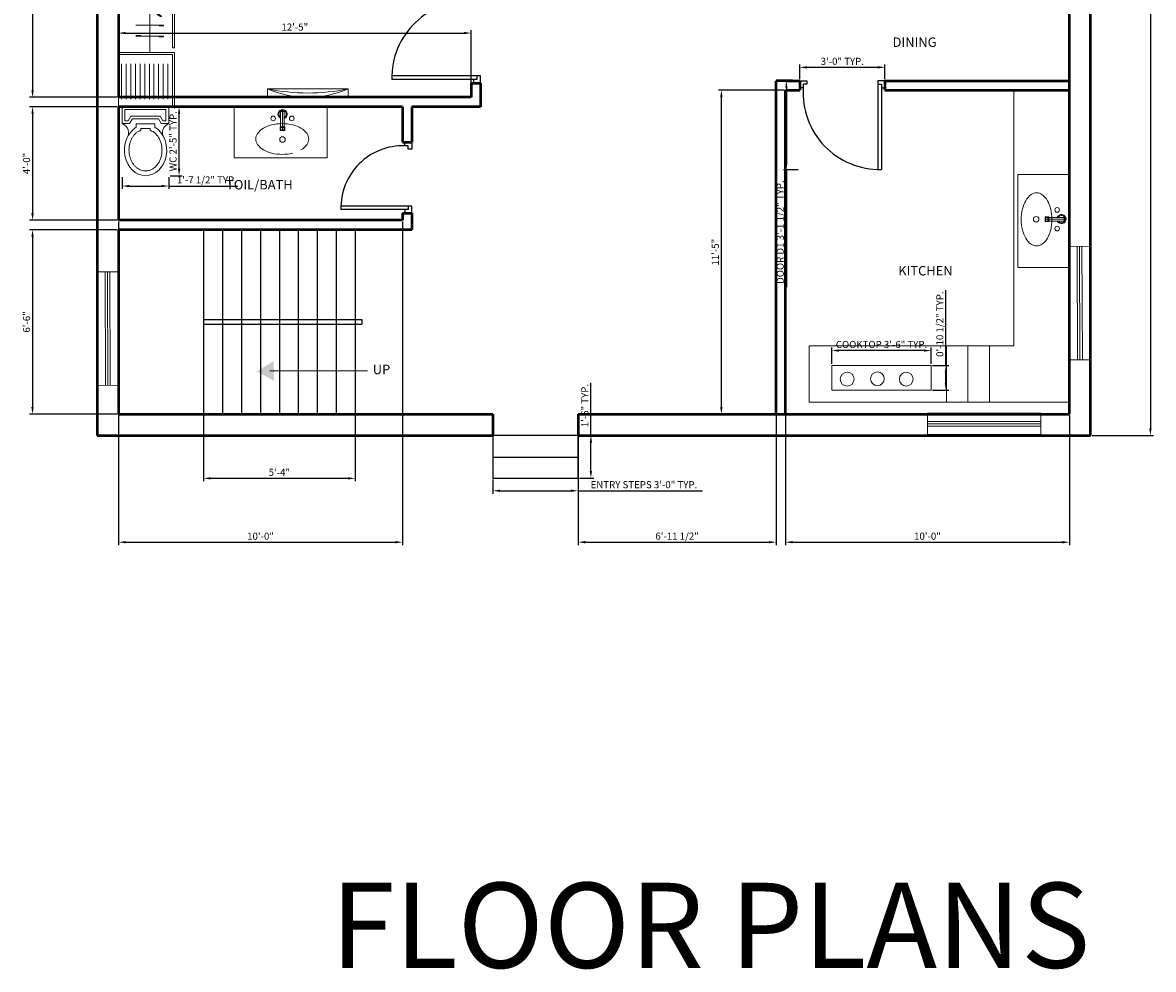
# Model space of a CAD drawing. Units: inches. Extents: x 108 to 1546, y -229 to 513.
# Tile 4 of 11: x 591 to 1070, y -229 to 171. Entities that reach past the tile are written whole.
import ezdxf

# ---------------------------------------------------------------- set-up
doc = ezdxf.new("R2010")
doc.units = ezdxf.units.IN
for name, color, linetype, lineweight in [('A-ANNO-DIMS', 2, 'Continuous', 18), ('A-ANNO-SYMB', 4, 'Continuous', 18), ('A-AREA-IDEN', 4, 'Continuous', 18), ('A-EQPM', 8, 'Continuous', 18), ('A-FLOR-CBNT', 8, 'Continuous', 18), ('A-FLOR-FIXT', 9, 'Continuous', 18), ('A-FLOR-STRS', 7, 'Continuous', 25), ('A-FURN', 8, 'Continuous', 13), ('door', 1, 'Continuous', 25), ('tv', 2, 'Continuous', 13), ('wall', 7, 'Continuous', 50), ('WINDOW', 212, 'Continuous', 18)]:
    doc.layers.add(name, color=color, linetype=linetype, lineweight=lineweight)
doc.layers.add('A-ANNO-TEXT', color=30, linetype='Continuous', lineweight=35, true_color=0xf26722)
doc.styles.get("Standard").update_dxf_attribs({"font": 'arial.ttf'})
doc.dimstyles.new('ISO-25', dxfattribs={"dimtxt": 3, "dimasz": 3, "dimexe": 1.25, "dimexo": 0.625, "dimtad": 1, "dimdec": 1, "dimlunit": 3, "dimtxsty": 'Standard', "dimcen": 2.5, "dimadec": 0, "dimazin": 0, "dimtfac": 1, "dimtdec": 1, "dimtmove": 0, "dimatfit": 3, "dimfxl": 1, "dimarcsym": 0})

# ---------------------------------------------------------------- blocks, each defined once
blk = doc.blocks.new('A$C50A015BB')
for p, q in [((0, 0.55), (1, 0.55)), ((0, 0.55), (0, 0)), ((0.498, 0.5), (0.538, 0.5)), ((0.498, 0.5), (0.498, 0.3)), ((0.518, 0.5), (0.518, 0.3)), ((0.538, 0.5), (0.538, 0.3)), ((1, 0.55), (1, 0)), ((0.493, 0.335), (0.493, 0.295)), ((0.493, 0.335), (0.543, 0.335)), ((0.493, 0.295), (0.543, 0.295)), ((0.498, 0.325), (0.538, 0.325)), ((0.498, 0.3), (0.538, 0.3)), ((0.543, 0.335), (0.543, 0.295)), ((0, 0), (1, 0)), ((0, 0), (1, 0))]:
    blk.add_line(p, q)
for centre, radius in [((0.418, 0.424), 0.025), ((0.618, 0.424), 0.025), ((0.518, 0.198), 0.0298)]:
    blk.add_circle(centre, radius)
for centre, radius, start, end in [((0.52, 0.47), 0.0497, 291.7425, 244.2331), ((0.52, 0.47), 0.0397, 297.632, 237.0256), ((0.516, -0.123), 0.491, 90, 103.4853), ((0.516, -0.123), 0.491, 76.5147, 90), ((0.33, 0.203), 0.0991, 144.4178, 180), ((0.418, 0.14), 0.208, 120.0686, 144.4178), ((0.477, 0.038), 0.325, 103.4853, 120.0686), ((0.554, 0.038), 0.325, 59.9314, 76.5147), ((0.613, 0.14), 0.208, 35.5822, 59.9314), ((0.702, 0.203), 0.0991, 0, 35.5822), ((0.33, 0.203), 0.0991, 180, 215.5822), ((0.418, 0.267), 0.208, 215.5822, 239.9314), ((0.613, 0.267), 0.208, 300.0686, 324.4178), ((0.702, 0.203), 0.0991, 324.4178, 0), ((0.477, 0.368), 0.325, 239.9314, 256.5147), ((0.516, 0.529), 0.491, 256.5147, 270), ((0.516, 0.529), 0.491, 270, 283.4853), ((0.554, 0.368), 0.325, 283.4853, 300.0686)]:
    blk.add_arc(centre, radius, start, end)
blk = doc.blocks.new('A$C7C8779AE')
for p, q in [((0, 0.74), (0, 0.56)), ((0.5, 0.74), (0, 0.74)), ((0.5, 0.56), (0.5, 0.74)), ((0.47, 0.71), (0.03, 0.71)), ((0.03, 0.71), (0.03, 0.59)), ((0.093, 0.64), (0.063, 0.59)), ((0.11, 0.61), (0.08, 0.56)), ((0.093, 0.64), (0.407, 0.64)), ((0.11, 0.61), (0.39, 0.61)), ((0.42, 0.56), (0.39, 0.61)), ((0.437, 0.59), (0.407, 0.64)), ((0.47, 0.59), (0.47, 0.71)), ((0, 0.56), (0.08, 0.56)), ((0.03, 0.59), (0.063, 0.59)), ((0.15, 0.557), (0.15, 0.52)), ((0.15, 0.557), (0.351, 0.557)), ((0.2, 0.507), (0.2, 0.488)), ((0.2, 0.507), (0.301, 0.507)), ((0.301, 0.507), (0.301, 0.488)), ((0.351, 0.557), (0.351, 0.52)), ((0.42, 0.56), (0.5, 0.56)), ((0.437, 0.59), (0.47, 0.59))]:
    blk.add_line(p, q)
for centre, start, end in [((-0.039, 0.461), 344.642, 68.7339), ((0.539, 0.461), 111.2661, 195.358)]:
    blk.add_arc(centre, 0.106, start, end)
blk.add_ellipse((0.251, 0.274), major_axis=(0, 0.274), ratio=0.828948, start_param=0.459479, end_param=5.823706)
blk.add_open_spline([(0.2, 0.488), (0.17, 0.474), (0.164, 0.47), (0.151, 0.46), (0.144, 0.454), (0.13, 0.439), (0.123, 0.431), (0.111, 0.413), (0.106, 0.404), (0.096, 0.384), (0.091, 0.373), (0.084, 0.352), (0.081, 0.34), (0.076, 0.317), (0.075, 0.305), (0.073, 0.282), (0.073, 0.27), (0.074, 0.246), (0.076, 0.234), (0.08, 0.211), (0.083, 0.2), (0.09, 0.178), (0.095, 0.167), (0.104, 0.147), (0.11, 0.138), (0.122, 0.12), (0.128, 0.112), (0.142, 0.097), (0.149, 0.09), (0.165, 0.078), (0.173, 0.073), (0.189, 0.064), (0.197, 0.06), (0.214, 0.055), (0.222, 0.053), (0.239, 0.05), (0.248, 0.05), (0.266, 0.051), (0.276, 0.052), (0.296, 0.057), (0.306, 0.061), (0.325, 0.071), (0.335, 0.077), (0.353, 0.091), (0.361, 0.099), (0.377, 0.117), (0.384, 0.127), (0.398, 0.149), (0.404, 0.161), (0.414, 0.185), (0.418, 0.198), (0.424, 0.225), (0.426, 0.239), (0.428, 0.267), (0.428, 0.281), (0.426, 0.309), (0.424, 0.323), (0.418, 0.349), (0.414, 0.363), (0.404, 0.387), (0.398, 0.399), (0.385, 0.421), (0.378, 0.431), (0.362, 0.449), (0.353, 0.458), (0.338, 0.469), (0.332, 0.474), (0.301, 0.488)], degree=3, knots=[0.459479, 0.459479, 0.459479, 0.459479, 0.567422, 0.567422, 0.720865, 0.720865, 0.874307, 0.874307, 1.02775, 1.02775, 1.181192, 1.181192, 1.334635, 1.334635, 1.488077, 1.488077, 1.64152, 1.64152, 1.794963, 1.794963, 1.948405, 1.948405, 2.101848, 2.101848, 2.25529, 2.25529, 2.408733, 2.408733, 2.562175, 2.562175, 2.715618, 2.715618, 2.86906, 2.86906, 3.022503, 3.022503, 3.175946, 3.175946, 3.356457, 3.356457, 3.536968, 3.536968, 3.717479, 3.717479, 3.89799, 3.89799, 4.078501, 4.078501, 4.259012, 4.259012, 4.439523, 4.439523, 4.620035, 4.620035, 4.800546, 4.800546, 4.981057, 4.981057, 5.161568, 5.161568, 5.342079, 5.342079, 5.52259, 5.52259, 5.703101, 5.703101, 5.823706, 5.823706, 5.823706, 5.823706])
blk = doc.blocks.new('A$C34930FF8')
at = {"ltscale": 0.05}
for p, q in [((0, 2252), (0, 17)), ((600, 2252), (0, 2252)), ((185, 1513), (185, 1521)), ((227, 1479), (233, 1485)), ((238, 1513), (238, 1521)), ((437, 1513), (437, 1504)), ((482, 1513), (482, 1504)), ((264, 1442), (270, 1448)), ((185, 1229), (185, 1238)), ((238, 1229), (238, 1238)), ((398, 1304), (392, 1298)), ((435, 1266), (429, 1260)), ((437, 1228), (437, 1220)), ((482, 1228), (482, 1220)), ((209, 1150), (214, 1157)), ((253, 1122), (258, 1129)), ((415, 1018), (411, 1010)), ((459, 989), (455, 982)), ((482, 895), (482, 886)), ((238, 775), (238, 784)), ((437, 775), (437, 767)), ((482, 775), (482, 767)), ((600, 17), (0, 17))]:
    blk.add_line(p, q, dxfattribs=at)
for p, q in [((580, 1691), (580, 2252)), ((600, 1669), (600, 2269)), ((30, 1791), (30, 2169)), ((80, 1791), (80, 2169)), ((130, 1791), (130, 2169)), ((180, 1791), (180, 2169)), ((230, 1791), (230, 2169)), ((280, 1791), (280, 2169)), ((330, 1791), (330, 2169)), ((380, 1791), (380, 2169)), ((430, 1791), (430, 2169)), ((480, 1791), (480, 2169)), ((530, 1791), (530, 2169)), ((580, 1691), (0, 1691)), ((600, 1669), (0, 1669)), ((335, 1666), (335, 603)), ((600, 1603), (620, 1603)), ((600, 1019), (600, 1603)), ((620, 1603), (620, 1019)), ((238, 1521), (185, 1521)), ((482, 1513), (185, 1513)), ((435, 1266), (227, 1479)), ((270, 1448), (233, 1485)), ((437, 1504), (482, 1504)), ((238, 1238), (185, 1238)), ((482, 1228), (185, 1228)), ((429, 1260), (392, 1298)), ((437, 1220), (482, 1220)), ((600, 1233), (580, 1233)), ((580, 1233), (580, 649)), ((600, 649), (600, 1233)), ((459, 989), (209, 1150)), ((258, 1129), (214, 1157)), ((455, 982), (411, 1010)), ((620, 1019), (600, 1019)), ((482, 895), (185, 895)), ((437, 886), (482, 886)), ((238, 784), (185, 784)), ((482, 775), (185, 775)), ((437, 767), (482, 767)), ((580, 649), (600, 649)), ((600, 600), (0, 600)), ((580, 578), (0, 578)), ((580, 578), (580, 17)), ((600, 600), (600, 0)), ((30, 478), (30, 100)), ((80, 478), (80, 100)), ((130, 478), (130, 100)), ((180, 478), (180, 100)), ((230, 478), (230, 100)), ((280, 478), (280, 100)), ((330, 478), (330, 100)), ((380, 478), (380, 100)), ((430, 478), (430, 100)), ((480, 478), (480, 100)), ((530, 478), (530, 100))]:
    blk.add_line(p, q)
blk = doc.blocks.new('*D24')
at = {"layer": 'A-ANNO-DIMS', "color": 0, "lineweight": -2, "transparency": 16777216}
for p, q in [((1043.62, 476.47), (1069.53, 476.47)), ((1068.28, 473.47), (1068.28, -0.53)), ((1043.62, -3.53), (1069.53, -3.53))]:
    blk.add_line(p, q, dxfattribs=at)
at = {"layer": 'A-ANNO-DIMS', "color": 0, "transparency": 16777216}
for points in [[(1067.78, 473.47), (1068.78, 473.47), (1068.28, 476.47)], [(1067.78, -0.53), (1068.78, -0.53), (1068.28, -3.53)]]:
    blk.add_solid(points, dxfattribs=at)
at = {"layer": 'Defpoints', "color": 0, "transparency": 16777216}
for p in [(1043, 476.47), (1043, -3.53), (1068.28, -3.53)]:
    blk.add_point(p, dxfattribs=at)
at = {"layer": 'A-ANNO-DIMS', "color": 0, "transparency": 16777216, "insert": (1066.12, 236.47), "char_height": 3, "attachment_point": 5, "rotation": 90}
blk.add_mtext("40'", dxfattribs=at)
blk = doc.blocks.new('WINDOW-48X9')
for p, q in [((0, 9), (0, 0)), ((0, 9), (48, 9)), ((0, 5.5), (48, 5.5)), ((48, 9), (48, 0)), ((0, 4.5), (48, 4.5)), ((0, 3.5), (48, 3.5)), ((0, 0), (48, 0))]:
    blk.add_line(p, q)
blk = doc.blocks.new('DOOR-SWING-36')
for p, q in [((1.5, 1.5), (1.5, 37.5)), ((3, 1.5), (3, 37.5)), ((0, 3), (0, 0)), ((1.5, 3), (0, 3)), ((1.5, 1.5), (1.5, 3)), ((3, 1.5), (1.5, 1.5)), ((3, 0), (3, 1.5)), ((33, 0), (33, 1.5)), ((33, 1.5), (34.5, 1.5)), ((34.5, 1.5), (34.5, 3)), ((34.5, 3), (36, 3)), ((36, 3), (36, 0)), ((0, 0), (3, 0)), ((36, 0), (33, 0))]:
    blk.add_line(p, q)
blk.add_arc((2.25, 5.18), 32.32, 356.1244, 91.3295)
blk = doc.blocks.new('DOOR-SWING-30')
for p, q in [((27, 30), (30, 30)), ((27, 28.5), (27, 30)), ((30, 30), (30, 27)), ((28.5, 28.5), (27, 28.5)), ((28.5, 27), (28.5, 28.5)), ((30, 27), (28.5, 27)), ((30, 3), (0, 3)), ((28.5, 1.5), (0, 1.5)), ((28.5, 1.5), (27, 1.5)), ((27, 1.5), (27, 0)), ((30, 3), (28.5, 3)), ((28.5, 3), (28.5, 1.5)), ((30, 0), (30, 3)), ((27, 0), (30, 0))]:
    blk.add_line(p, q)
blk.add_arc((26.25, 2.25), 26.26, 88.3634, 181.6366)
blk = doc.blocks.new('TV-WALL-MOUNT')
blk.add_lwpolyline([(0, 0), (34.19, 0), (34.19, 3.56), (0, 3.56)], close=True)
for centre, radius, start, end in [((17.1, 42.8), 42.8, 246.4582, 293.5418), ((17.1, 84.72), 82.93, 258.1036, 281.8964)]:
    blk.add_arc(centre, radius, start, end)
blk = doc.blocks.new('COOKTOP-3-BURNER')
blk.add_lwpolyline([(0, 41.89), (10.48, 41.89), (10.48, 0), (0, 0)], close=True)
for centre in [(4.66, 35.46), (4.81, 22.66), (4.66, 10.45)]:
    blk.add_circle(centre, 2.9)
blk = doc.blocks.new('COUNTER-INSERT-DIVIDED')
blk.add_line((0, 9.14), (23.96, 9.14))
blk.add_lwpolyline([(0, 18.28), (23.96, 18.28), (23.96, 0), (0, 0)], close=True)
blk = doc.blocks.new('ENTRY-STEPS-36')
for p, q in [((0, 8.79), (36, 8.79)), ((0, 0), (36, 0))]:
    blk.add_line(p, q)
blk.add_lwpolyline([(36, 0), (36, 18), (0, 18), (0, 0)])
blk = doc.blocks.new('*D38')
at = {"layer": 'A-ANNO-DIMS', "color": 0, "lineweight": -2, "transparency": 16777216}
for p, q in [((919.37, 146.47), (913.09, 146.47)), ((914.34, 143.47), (914.34, 111.76)), ((919.37, 108.76), (913.09, 108.76)), ((914.34, 108.76), (914.34, 59.12))]:
    blk.add_line(p, q, dxfattribs=at)
at = {"layer": 'A-ANNO-DIMS', "color": 0, "transparency": 16777216}
for points in [[(913.84, 143.47), (914.84, 143.47), (914.34, 146.47)], [(913.84, 111.76), (914.84, 111.76), (914.34, 108.76)]]:
    blk.add_solid(points, dxfattribs=at)
at = {"layer": 'Defpoints', "color": 0, "transparency": 16777216}
for p in [(920, 146.47), (914.34, 108.76), (920, 108.76)]:
    blk.add_point(p, dxfattribs=at)
at = {"layer": 'A-ANNO-DIMS', "color": 0, "transparency": 16777216, "insert": (912.16, 82.44), "char_height": 3, "attachment_point": 5, "rotation": 90}
blk.add_mtext('DOOR D1 3\'-1 1/2" TYP.', dxfattribs=at)
blk = doc.blocks.new('*D39')
at = {"layer": 'A-ANNO-DIMS', "color": 0, "lineweight": -2, "transparency": 16777216}
for p, q in [((920, 147.09), (920, 153.38)), ((956, 147.09), (956, 153.38)), ((953, 152.13), (923, 152.13))]:
    blk.add_line(p, q, dxfattribs=at)
at = {"layer": 'A-ANNO-DIMS', "color": 0, "transparency": 16777216}
for points in [[(923, 152.63), (923, 151.63), (920, 152.13)], [(953, 152.63), (953, 151.63), (956, 152.13)]]:
    blk.add_solid(points, dxfattribs=at)
at = {"layer": 'Defpoints', "color": 0, "transparency": 16777216}
for p in [(920, 152.13), (920, 146.47), (956, 146.47)]:
    blk.add_point(p, dxfattribs=at)
at = {"layer": 'A-ANNO-DIMS', "color": 0, "transparency": 16777216, "insert": (938, 154.28), "char_height": 3, "attachment_point": 5}
blk.add_mtext('3\'-0" TYP.', dxfattribs=at)
blk = doc.blocks.new('*D48')
at = {"layer": 'A-ANNO-DIMS', "color": 0, "lineweight": -2, "transparency": 16777216}
for p, q in [((653.82, 135.47), (658.82, 135.47)), ((657.57, 109.32), (657.57, 132.47)), ((653.82, 106.32), (658.82, 106.32))]:
    blk.add_line(p, q, dxfattribs=at)
at = {"layer": 'A-ANNO-DIMS', "color": 0, "transparency": 16777216}
for points in [[(657.07, 132.47), (658.07, 132.47), (657.57, 135.47)], [(657.07, 109.32), (658.07, 109.32), (657.57, 106.32)]]:
    blk.add_solid(points, dxfattribs=at)
at = {"layer": 'Defpoints', "color": 0, "transparency": 16777216}
for p in [(653.2, 135.47), (657.57, 135.47), (653.2, 106.32)]:
    blk.add_point(p, dxfattribs=at)
at = {"layer": 'A-ANNO-DIMS', "color": 0, "transparency": 16777216, "insert": (655.4, 120.89), "char_height": 3, "attachment_point": 5, "rotation": 90}
blk.add_mtext('WC 2\'-5" TYP.', dxfattribs=at)
blk = doc.blocks.new('*D49')
at = {"layer": 'A-ANNO-DIMS', "color": 0, "lineweight": -2, "transparency": 16777216}
for p, q in [((633.51, 105.69), (633.51, 100.7)), ((653.2, 105.69), (653.2, 100.7)), ((636.51, 101.95), (650.2, 101.95)), ((653.2, 101.95), (682.44, 101.95))]:
    blk.add_line(p, q, dxfattribs=at)
at = {"layer": 'A-ANNO-DIMS', "color": 0, "transparency": 16777216}
for points in [[(636.51, 102.45), (636.51, 101.45), (633.51, 101.95)], [(650.2, 102.45), (650.2, 101.45), (653.2, 101.95)]]:
    blk.add_solid(points, dxfattribs=at)
at = {"layer": 'Defpoints', "color": 0, "transparency": 16777216}
for p in [(633.51, 106.32), (653.2, 106.32), (653.2, 101.95)]:
    blk.add_point(p, dxfattribs=at)
at = {"layer": 'A-ANNO-DIMS', "color": 0, "transparency": 16777216, "insert": (669.32, 104.12), "char_height": 3, "attachment_point": 5}
blk.add_mtext('1\'-7 1/2" TYP.', dxfattribs=at)
blk = doc.blocks.new('*D62')
at = {"layer": 'A-ANNO-DIMS', "color": 0, "lineweight": -2, "transparency": 16777216}
for p, q in [((933.62, 26.71), (933.62, 33.62)), ((975.51, 26.71), (975.51, 33.62)), ((972.51, 32.37), (936.62, 32.37))]:
    blk.add_line(p, q, dxfattribs=at)
at = {"layer": 'A-ANNO-DIMS', "color": 0, "transparency": 16777216}
for points in [[(936.62, 32.87), (936.62, 31.87), (933.62, 32.37)], [(972.51, 32.87), (972.51, 31.87), (975.51, 32.37)]]:
    blk.add_solid(points, dxfattribs=at)
at = {"layer": 'Defpoints', "color": 0, "transparency": 16777216}
for p in [(933.62, 32.37), (933.62, 26.09), (975.51, 26.09)]:
    blk.add_point(p, dxfattribs=at)
at = {"layer": 'A-ANNO-DIMS', "color": 0, "transparency": 16777216, "insert": (954.57, 34.55), "char_height": 3, "attachment_point": 5}
blk.add_mtext('COOKTOP 3\'-6" TYP.', dxfattribs=at)
blk = doc.blocks.new('*D63')
at = {"layer": 'A-ANNO-DIMS', "color": 0, "lineweight": -2, "transparency": 16777216}
for p, q in [((981.8, 26.09), (981.8, 57.95)), ((976.14, 26.09), (983.05, 26.09)), ((981.8, 18.61), (981.8, 23.09)), ((976.14, 15.61), (983.05, 15.61))]:
    blk.add_line(p, q, dxfattribs=at)
at = {"layer": 'A-ANNO-DIMS', "color": 0, "transparency": 16777216}
for points in [[(981.3, 23.09), (982.3, 23.09), (981.8, 26.09)], [(981.3, 18.61), (982.3, 18.61), (981.8, 15.61)]]:
    blk.add_solid(points, dxfattribs=at)
at = {"layer": 'Defpoints', "color": 0, "transparency": 16777216}
for p in [(975.51, 26.09), (981.8, 26.09), (975.51, 15.61)]:
    blk.add_point(p, dxfattribs=at)
at = {"layer": 'A-ANNO-DIMS', "color": 0, "transparency": 16777216, "insert": (979.62, 43.52), "char_height": 3, "attachment_point": 5, "rotation": 90}
blk.add_mtext('0\'-10 1/2" TYP.', dxfattribs=at)
blk = doc.blocks.new('*D66')
at = {"layer": 'A-ANNO-DIMS', "color": 0, "lineweight": -2, "transparency": 16777216}
for p, q in [((790.29, -22.16), (790.29, -28.18)), ((826.29, -22.16), (826.29, -28.18)), ((793.29, -26.93), (823.29, -26.93)), ((826.29, -26.93), (878.94, -26.93))]:
    blk.add_line(p, q, dxfattribs=at)
at = {"layer": 'A-ANNO-DIMS', "color": 0, "transparency": 16777216}
for points in [[(793.29, -26.43), (793.29, -27.43), (790.29, -26.93)], [(823.29, -26.43), (823.29, -27.43), (826.29, -26.93)]]:
    blk.add_solid(points, dxfattribs=at)
at = {"layer": 'Defpoints', "color": 0, "transparency": 16777216}
for p in [(790.29, -21.53), (826.29, -21.53), (826.29, -26.93)]:
    blk.add_point(p, dxfattribs=at)
at = {"layer": 'A-ANNO-DIMS', "color": 0, "transparency": 16777216, "insert": (854.11, -24.75), "char_height": 3, "attachment_point": 5}
blk.add_mtext('ENTRY STEPS 3\'-0" TYP.', dxfattribs=at)
blk = doc.blocks.new('*D67')
at = {"layer": 'A-ANNO-DIMS', "color": 0, "lineweight": -2, "transparency": 16777216}
for p, q in [((831.69, -3.53), (831.69, 18.72)), ((826.91, -3.53), (832.94, -3.53)), ((831.69, -18.53), (831.69, -6.53)), ((826.91, -21.53), (832.94, -21.53))]:
    blk.add_line(p, q, dxfattribs=at)
at = {"layer": 'A-ANNO-DIMS', "color": 0, "transparency": 16777216}
for points in [[(831.19, -6.53), (832.19, -6.53), (831.69, -3.53)], [(831.19, -18.53), (832.19, -18.53), (831.69, -21.53)]]:
    blk.add_solid(points, dxfattribs=at)
at = {"layer": 'Defpoints', "color": 0, "transparency": 16777216}
for p in [(826.29, -3.53), (831.69, -3.53), (826.29, -21.53)]:
    blk.add_point(p, dxfattribs=at)
at = {"layer": 'A-ANNO-DIMS', "color": 0, "transparency": 16777216, "insert": (829.53, 9.1), "char_height": 3, "attachment_point": 5, "rotation": 90}
blk.add_mtext('1\'-6" TYP.', dxfattribs=at)
blk = doc.blocks.new('*D87')
at = {"layer": 'A-ANNO-DIMS', "color": 0, "lineweight": -2, "transparency": 16777216}
for p, q in [((632, 86.84), (632, -49.93)), ((752, 86.84), (752, -49.93)), ((635, -48.68), (749, -48.68))]:
    blk.add_line(p, q, dxfattribs=at)
at = {"layer": 'A-ANNO-DIMS', "color": 0, "transparency": 16777216}
for points in [[(635, -48.18), (635, -49.18), (632, -48.68)], [(749, -48.18), (749, -49.18), (752, -48.68)]]:
    blk.add_solid(points, dxfattribs=at)
at = {"layer": 'Defpoints', "color": 0, "transparency": 16777216}
for p in [(632, 87.47), (752, 87.47), (752, -48.68)]:
    blk.add_point(p, dxfattribs=at)
at = {"layer": 'A-ANNO-DIMS', "color": 0, "transparency": 16777216, "insert": (692, -46.52), "char_height": 3, "attachment_point": 5}
blk.add_mtext('10\'-0"', dxfattribs=at)
blk = doc.blocks.new('*D88')
at = {"layer": 'A-ANNO-DIMS', "color": 0, "lineweight": -2, "transparency": 16777216}
for p, q in [((632, 140.09), (632, 167.87)), ((781, 140.09), (781, 167.87)), ((635, 166.62), (778, 166.62))]:
    blk.add_line(p, q, dxfattribs=at)
at = {"layer": 'A-ANNO-DIMS', "color": 0, "transparency": 16777216}
for points in [[(635, 167.12), (635, 166.12), (632, 166.62)], [(778, 167.12), (778, 166.12), (781, 166.62)]]:
    blk.add_solid(points, dxfattribs=at)
at = {"layer": 'Defpoints', "color": 0, "transparency": 16777216}
for p in [(781, 166.62), (632, 139.47), (781, 139.47)]:
    blk.add_point(p, dxfattribs=at)
at = {"layer": 'A-ANNO-DIMS', "color": 0, "transparency": 16777216, "insert": (706.5, 168.78), "char_height": 3, "attachment_point": 5}
blk.add_mtext('12\'-5"', dxfattribs=at)
blk = doc.blocks.new('*D89')
at = {"layer": 'A-ANNO-DIMS', "color": 0, "lineweight": -2, "transparency": 16777216}
for p, q in [((914, 4.84), (914, -49.93)), ((1034, 4.84), (1034, -49.93)), ((917, -48.68), (1031, -48.68))]:
    blk.add_line(p, q, dxfattribs=at)
at = {"layer": 'A-ANNO-DIMS', "color": 0, "transparency": 16777216}
for points in [[(917, -48.18), (917, -49.18), (914, -48.68)], [(1031, -48.18), (1031, -49.18), (1034, -48.68)]]:
    blk.add_solid(points, dxfattribs=at)
at = {"layer": 'Defpoints', "color": 0, "transparency": 16777216}
for p in [(914, 5.47), (1034, 5.47), (1034, -48.68)]:
    blk.add_point(p, dxfattribs=at)
at = {"layer": 'A-ANNO-DIMS', "color": 0, "transparency": 16777216, "insert": (974, -46.52), "char_height": 3, "attachment_point": 5}
blk.add_mtext('10\'-0"', dxfattribs=at)
blk = doc.blocks.new('*D90')
at = {"layer": 'A-ANNO-DIMS', "color": 0, "lineweight": -2, "transparency": 16777216}
for p, q in [((910, 4.84), (910, -49.93)), ((826.29, -4.16), (826.29, -49.93)), ((829.29, -48.68), (907, -48.68))]:
    blk.add_line(p, q, dxfattribs=at)
at = {"layer": 'A-ANNO-DIMS', "color": 0, "transparency": 16777216}
for points in [[(829.29, -48.18), (829.29, -49.18), (826.29, -48.68)], [(907, -48.18), (907, -49.18), (910, -48.68)]]:
    blk.add_solid(points, dxfattribs=at)
at = {"layer": 'Defpoints', "color": 0, "transparency": 16777216}
for p in [(910, 5.47), (826.29, -3.53), (910, -48.68)]:
    blk.add_point(p, dxfattribs=at)
at = {"layer": 'A-ANNO-DIMS', "color": 0, "transparency": 16777216, "insert": (868.14, -46.5), "char_height": 3, "attachment_point": 5}
blk.add_mtext('6\'-11 1/2"', dxfattribs=at)
blk = doc.blocks.new('*D93')
at = {"layer": 'A-ANNO-DIMS', "color": 0, "lineweight": -2, "transparency": 16777216}
for p, q in [((631.37, 307.47), (594.36, 307.47)), ((595.61, 304.47), (595.61, 142.47)), ((631.37, 139.47), (594.36, 139.47))]:
    blk.add_line(p, q, dxfattribs=at)
at = {"layer": 'A-ANNO-DIMS', "color": 0, "transparency": 16777216}
for points in [[(595.11, 304.47), (596.11, 304.47), (595.61, 307.47)], [(595.11, 142.47), (596.11, 142.47), (595.61, 139.47)]]:
    blk.add_solid(points, dxfattribs=at)
at = {"layer": 'Defpoints', "color": 0, "transparency": 16777216}
for p in [(632, 307.47), (595.61, 139.47), (632, 139.47)]:
    blk.add_point(p, dxfattribs=at)
at = {"layer": 'A-ANNO-DIMS', "color": 0, "transparency": 16777216, "insert": (593.45, 223.47), "char_height": 3, "attachment_point": 5, "rotation": 90}
blk.add_mtext('14\'-0"', dxfattribs=at)
blk = doc.blocks.new('*D94')
at = {"layer": 'A-ANNO-DIMS', "color": 0, "lineweight": -2, "transparency": 16777216}
for p, q in [((631.37, 135.47), (594.36, 135.47)), ((595.61, 132.47), (595.61, 90.47)), ((631.37, 87.47), (594.36, 87.47))]:
    blk.add_line(p, q, dxfattribs=at)
at = {"layer": 'A-ANNO-DIMS', "color": 0, "transparency": 16777216}
for points in [[(595.11, 132.47), (596.11, 132.47), (595.61, 135.47)], [(595.11, 90.47), (596.11, 90.47), (595.61, 87.47)]]:
    blk.add_solid(points, dxfattribs=at)
at = {"layer": 'Defpoints', "color": 0, "transparency": 16777216}
for p in [(632, 135.47), (595.61, 87.47), (632, 87.47)]:
    blk.add_point(p, dxfattribs=at)
at = {"layer": 'A-ANNO-DIMS', "color": 0, "transparency": 16777216, "insert": (593.45, 111.47), "char_height": 3, "attachment_point": 5, "rotation": 90}
blk.add_mtext('4\'-0"', dxfattribs=at)
blk = doc.blocks.new('*D95')
at = {"layer": 'A-ANNO-DIMS', "color": 0, "lineweight": -2, "transparency": 16777216}
for p, q in [((631.37, 83.47), (594.36, 83.47)), ((595.61, 80.47), (595.61, 8.47)), ((631.37, 5.47), (594.36, 5.47))]:
    blk.add_line(p, q, dxfattribs=at)
at = {"layer": 'A-ANNO-DIMS', "color": 0, "transparency": 16777216}
for points in [[(595.11, 80.47), (596.11, 80.47), (595.61, 83.47)], [(595.11, 8.47), (596.11, 8.47), (595.61, 5.47)]]:
    blk.add_solid(points, dxfattribs=at)
at = {"layer": 'Defpoints', "color": 0, "transparency": 16777216}
for p in [(632, 83.47), (595.61, 5.47), (632, 5.47)]:
    blk.add_point(p, dxfattribs=at)
at = {"layer": 'A-ANNO-DIMS', "color": 0, "transparency": 16777216, "insert": (593.45, 44.47), "char_height": 3, "attachment_point": 5, "rotation": 90}
blk.add_mtext('6\'-6"', dxfattribs=at)
blk = doc.blocks.new('*D96')
at = {"layer": 'A-ANNO-DIMS', "color": 0, "lineweight": -2, "transparency": 16777216}
for p, q in [((913.37, 142.47), (885.6, 142.47)), ((886.85, 8.47), (886.85, 139.47)), ((913.37, 5.47), (885.6, 5.47))]:
    blk.add_line(p, q, dxfattribs=at)
at = {"layer": 'A-ANNO-DIMS', "color": 0, "transparency": 16777216}
for points in [[(886.35, 139.47), (887.35, 139.47), (886.85, 142.47)], [(886.35, 8.47), (887.35, 8.47), (886.85, 5.47)]]:
    blk.add_solid(points, dxfattribs=at)
at = {"layer": 'Defpoints', "color": 0, "transparency": 16777216}
for p in [(886.85, 142.47), (914, 142.47), (914, 5.47)]:
    blk.add_point(p, dxfattribs=at)
at = {"layer": 'A-ANNO-DIMS', "color": 0, "transparency": 16777216, "insert": (884.69, 73.97), "char_height": 3, "attachment_point": 5, "rotation": 90}
blk.add_mtext('11\'-5"', dxfattribs=at)
blk = doc.blocks.new('*D98')
at = {"layer": 'A-ANNO-DIMS', "color": 0, "lineweight": -2, "transparency": 16777216}
for p, q in [((667.96, 4.84), (667.96, -22.93)), ((731.96, 4.84), (731.96, -22.93)), ((728.96, -21.68), (670.96, -21.68))]:
    blk.add_line(p, q, dxfattribs=at)
at = {"layer": 'A-ANNO-DIMS', "color": 0, "transparency": 16777216}
for points in [[(670.96, -21.18), (670.96, -22.18), (667.96, -21.68)], [(728.96, -21.18), (728.96, -22.18), (731.96, -21.68)]]:
    blk.add_solid(points, dxfattribs=at)
at = {"layer": 'Defpoints', "color": 0, "transparency": 16777216}
for p in [(667.96, 5.47), (731.96, 5.47), (667.96, -21.68)]:
    blk.add_point(p, dxfattribs=at)
at = {"layer": 'A-ANNO-DIMS', "color": 0, "transparency": 16777216, "insert": (699.96, -19.53), "char_height": 3, "attachment_point": 5}
blk.add_mtext('5\'-4"', dxfattribs=at)

msp = doc.modelspace()

# ---------------------------------------------------------------- hatches: boundary and pattern name
at = {"layer": 'A-ANNO-SYMB'}
h = msp.add_hatch(color=256, dxfattribs=at)
h.dxf.hatch_style = 1
h.paths.add_polyline_path([(697.54, 27.91), (690.43, 23.51), (693.27, 21.98), (697.65, 24.4)])
h.paths.add_polyline_path([(697.65, 24.4), (693.27, 21.98), (697.79, 19.55)])

# ---------------------------------------------------------------- linework, layer by layer
msp.add_line((737.23, 23.79), (695.97, 23.79), dxfattribs=at)
at = {"layer": 'A-FLOR-CBNT'}
for p, q in [((1034, 142.47), (1010.56, 142.47)), ((1010.56, 142.47), (1010.56, 34.43)), ((1034, 10.47), (1034, 142.47)), ((924, 10.47), (924, 34.43)), ((924, 34.43), (1010.56, 34.43)), ((1034, 10.47), (924, 10.47))]:
    msp.add_line(p, q, dxfattribs=at)
at = {"layer": 'A-FLOR-FIXT'}
for p, q in [((680.87, 135.48), (720.24, 135.48)), ((680.87, 135.48), (680.87, 113.83)), ((720.24, 135.48), (720.24, 113.83)), ((700.49, 133.51), (702.07, 133.51)), ((700.49, 133.51), (700.49, 125.64)), ((701.28, 133.51), (701.28, 125.64)), ((702.07, 133.51), (702.07, 125.64)), ((700.3, 127.02), (700.3, 125.44)), ((700.3, 127.02), (702.27, 127.02)), ((700.3, 125.44), (702.27, 125.44)), ((700.49, 126.62), (702.07, 126.62)), ((700.49, 125.64), (702.07, 125.64)), ((702.27, 127.02), (702.27, 125.44)), ((680.87, 113.83), (720.24, 113.83)), ((680.87, 113.83), (720.24, 113.83))]:
    msp.add_line(p, q, dxfattribs=at)
for centre, radius in [((697.34, 130.52), 0.984), ((705.22, 130.52), 0.984), ((701.28, 121.63), 1.17)]:
    msp.add_circle(centre, radius, dxfattribs=at)
for centre, radius, start, end in [((701.34, 132.34), 1.96, 291.7425, 244.2331), ((701.34, 132.34), 1.56, 297.632, 237.0256), ((697.35, 119.33), 8.19, 120.0686, 144.4178), ((699.66, 115.34), 12.8, 103.4853, 120.0686), ((701.17, 109), 19.32, 90, 103.4853), ((701.17, 109), 19.32, 76.5147, 90), ((702.69, 115.34), 12.8, 59.9314, 76.5147), ((705, 119.33), 8.19, 35.5822, 59.9314), ((693.86, 121.82), 3.9, 144.4178, 180), ((693.86, 121.82), 3.9, 180, 215.5822), ((697.35, 124.32), 8.19, 215.5822, 239.9314), ((705, 124.32), 8.19, 300.0686, 324.4178), ((708.49, 121.82), 3.9, 0, 35.5822), ((708.49, 121.82), 3.9, 324.4178, 0), ((699.66, 128.31), 12.8, 239.9314, 256.5147), ((701.17, 134.64), 19.32, 256.5147, 270), ((701.17, 134.64), 19.32, 270, 283.4853)]:
    msp.add_arc(centre, radius, start, end, dxfattribs=at)
at = {"layer": 'A-FLOR-STRS'}
for p, q in [((632, 83.47), (667.96, 83.47)), ((632, 5.47), (632, 83.47)), ((667.96, 83.47), (667.96, 5.47)), ((675.96, 83.47), (675.96, 5.47)), ((683.96, 83.47), (683.96, 5.47)), ((691.96, 83.47), (691.96, 5.47)), ((699.96, 83.47), (699.96, 5.47)), ((707.96, 83.47), (707.96, 5.47)), ((715.96, 83.47), (715.96, 5.47)), ((723.96, 83.47), (723.96, 5.47)), ((731.96, 83.47), (731.96, 5.47)), ((667.96, 45.47), (734.83, 45.47)), ((667.96, 43.47), (734.83, 43.47)), ((734.83, 45.47), (734.83, 43.47)), ((667.96, 5.47), (632, 5.47))]:
    msp.add_line(p, q, dxfattribs=at)
at = {"layer": 'wall'}
for p, q in [((623, 476.47), (623, -3.53)), ((1043, -3.53), (1043, 476.47)), ((1034, 5.47), (1034, 467.47)), ((632, 307.47), (632, 139.47)), ((781, 145.47), (785, 145.47)), ((781, 145.47), (781, 139.47)), ((785, 145.47), (785, 135.47)), ((910, 5.47), (910, 146.47)), ((917, 146.47), (910, 146.47)), ((914, 146.47), (920, 146.47)), ((920, 146.47), (920, 142.47)), ((956, 146.47), (956, 142.47)), ((956, 146.47), (1034, 146.47)), ((781, 139.47), (632, 139.47)), ((914, 5.47), (914, 142.47)), ((914, 142.47), (920, 142.47)), ((956, 142.47), (1034, 142.47)), ((752, 135.47), (632, 135.47)), ((632, 135.47), (632, 87.47)), ((752, 135.47), (752, 120.47)), ((756, 135.47), (756, 120.47)), ((785, 135.47), (756, 135.47)), ((752, 120.47), (756, 120.47)), ((752, 87.47), (632, 87.47)), ((752, 90.47), (756, 90.47)), ((752, 90.47), (752, 87.47)), ((756, 90.47), (756, 83.47)), ((756, 83.47), (632, 83.47)), ((632, 83.47), (632, 5.47)), ((632, 5.47), (790.29, 5.47)), ((790.29, 5.47), (790.29, -3.53)), ((826.29, 5.47), (826.29, -3.53)), ((826.29, 5.47), (1034, 5.47)), ((623, -3.53), (790.29, -3.53)), ((826.29, -3.53), (1043, -3.53))]:
    msp.add_line(p, q, dxfattribs=at)

# ---------------------------------------------------------------- block references
at = {"layer": 'A-EQPM', "rotation": 90.00000000000006}
msp.add_blockref('COOKTOP-3-BURNER', (975.51, 15.61), dxfattribs=at)
at = {"layer": 'A-FLOR-CBNT', "rotation": 90.00000000000063}
msp.add_blockref('COUNTER-INSERT-DIVIDED', (1000.28, 10.47), dxfattribs=at)
at = {"layer": 'A-FLOR-FIXT', "xscale": 39.37007874015748, "yscale": 39.37007874015748, "zscale": 39.37007874015748}
msp.add_blockref('A$C7C8779AE', (633.51, 106.32), dxfattribs=at)
at = {"layer": 'A-FLOR-FIXT', "xscale": -39.37007874015748, "yscale": 39.37007874015748, "zscale": 39.37007874015748, "rotation": 270}
msp.add_blockref('A$C50A015BB', (1012.15, 67.5), dxfattribs=at)
at = {"layer": 'A-FLOR-STRS'}
msp.add_blockref('ENTRY-STEPS-36', (790.29, -21.53), dxfattribs=at)
at = {"layer": 'A-FURN', "xscale": 0.0393700787401575, "yscale": 0.0393700787401575, "zscale": 0.0393700787401575}
msp.add_blockref('A$C34930FF8', (632, 134.79), dxfattribs=at)
at = {"layer": 'door'}
for p, rotation in [((785, 145.47), 90.00000000000031), ((956, 146.47), 180)]:
    msp.add_blockref('DOOR-SWING-36', p, dxfattribs=dict(at, rotation=rotation))
msp.add_blockref('DOOR-SWING-30', (725.99, 90.47), dxfattribs=at)
at = {"layer": 'tv'}
msp.add_blockref('TV-WALL-MOUNT', (694.9, 139.47), dxfattribs=at)
at = {"layer": 'WINDOW'}
for p, rotation in [((1042.99, 28.47), 90.2799560098102), ((631.99, 17.69), 90.27995600981046), ((1021.99, 5.92), 180)]:
    msp.add_blockref('WINDOW-48X9', p, dxfattribs=dict(at, rotation=rotation))

# ---------------------------------------------------------------- texts
at = {"layer": 'A-ANNO-SYMB', "insert": (739.46, 26.36), "char_height": 4, "attachment_point": 1}
msp.add_mtext_dynamic_manual_height_columns('UP', width=57.4311, gutter_width=12.5, heights=[12.84], dxfattribs=at)
at = {"layer": 'A-ANNO-TEXT', "insert": (721.58, -192.69), "char_height": 36, "attachment_point": 1}
msp.add_mtext_dynamic_manual_height_columns('FLOOR PLANS', width=662.4992, gutter_width=12.5, heights=[0], dxfattribs=at)
at = {"layer": 'A-AREA-IDEN', "char_height": 4, "attachment_point": 1}
for s, insert in [('DINING', (959.25, 164.76)), ('TOIL/BATH', (677.44, 104.49)), ('KITCHEN', (961.64, 68.12))]:
    msp.add_mtext_dynamic_manual_height_columns(s, width=57.4311, gutter_width=12.5, heights=[12.84], dxfattribs=dict(at, insert=insert))

# ---------------------------------------------------------------- dimensions: what is measured, and where the dimension line sits
at = {"layer": 'A-ANNO-DIMS'}
for base, p1, p2, angle, override, picture, middle in [((1068.28, -3.53), (1043, 476.47), (1043, -3.53), 90, {"dimclrd": 0, "dimclre": 0, "dimclrt": 0}, '*D24', (1066.12, 236.47)), ((595.61, 139.47), (632, 307.47), (632, 139.47), 90, {"dimdec": 1, "dimlfac": 1, "dimrnd": 0, "dimzin": 1, "dimdsep": 46, "dimlunit": 4, "dimfrac": 2}, '*D93', (593.45, 223.47)), ((886.85, 142.47), (914, 5.47), (914, 142.47), 90, {"dimdec": 1, "dimlfac": 1, "dimrnd": 0, "dimzin": 1, "dimdsep": 46, "dimlunit": 4, "dimfrac": 2}, '*D96', (884.69, 73.97)), ((595.61, 87.47), (632, 135.47), (632, 87.47), 90, {"dimdec": 1, "dimlfac": 1, "dimrnd": 0, "dimzin": 1, "dimdsep": 46, "dimlunit": 4, "dimfrac": 2}, '*D94', (593.45, 111.47)), ((595.61, 5.47), (632, 83.47), (632, 5.47), 90, {"dimdec": 1, "dimlfac": 1, "dimrnd": 0, "dimzin": 1, "dimdsep": 46, "dimlunit": 4, "dimfrac": 2}, '*D95', (593.45, 44.47)), ((667.96, -21.68), (731.96, 5.47), (667.96, 5.47), 180, {"dimdec": 1, "dimlfac": 1, "dimrnd": 0, "dimzin": 1, "dimdsep": 46, "dimlunit": 4, "dimfrac": 2}, '*D98', (699.96, -19.53))]:
    dim = msp.add_linear_dim(base=base, p1=p1, p2=p2, angle=angle, dimstyle='ISO-25', override=override, dxfattribs=at)
    dim.commit()
    dim.dimension.update_dxf_attribs({"geometry": picture, "text_midpoint": middle})
for base, p1, p2, picture, middle in [((781, 166.62), (632, 139.47), (781, 139.47), '*D88', (706.5, 168.78)), ((752, -48.68), (632, 87.47), (752, 87.47), '*D87', (692, -46.52)), ((910, -48.68), (826.29, -3.53), (910, 5.47), '*D90', (868.14, -46.5)), ((1034, -48.68), (914, 5.47), (1034, 5.47), '*D89', (974, -46.52))]:
    dim = msp.add_linear_dim(base=base, p1=p1, p2=p2, dimstyle='ISO-25', override={"dimdec": 1, "dimlfac": 1, "dimrnd": 0, "dimzin": 1, "dimdsep": 46, "dimlunit": 4, "dimfrac": 2}, dxfattribs=at)
    dim.commit()
    dim.dimension.update_dxf_attribs({"geometry": picture, "text_midpoint": middle})
for base, p1, p2, angle, text, picture, middle in [((920, 152.13), (956, 146.47), (920, 146.47), 180, '<> TYP.', '*D39', (938, 154.28)), ((914.34, 108.76), (920, 146.47), (920, 108.76), 270, 'DOOR D1 <> TYP.', '*D38', (912.16, 82.44)), ((657.5718, 135.4699), (653.199, 106.3178), (653.199, 135.4699), 90, 'WC <> TYP.', '*D48', (655.3956, 120.8939)), ((981.8, 26.09), (975.51, 15.61), (975.51, 26.09), 90, '<> TYP.', '*D63', (979.62, 43.52)), ((933.62, 32.37), (975.51, 26.09), (933.62, 26.09), 180, 'COOKTOP <> TYP.', '*D62', (954.57, 34.55)), ((831.69, -3.53), (826.29, -21.53), (826.29, -3.53), 90, '<> TYP.', '*D67', (829.53, 9.1))]:
    dim = msp.add_linear_dim(base=base, p1=p1, p2=p2, angle=angle, text=text, dimstyle='ISO-25', override={"dimdec": 1, "dimlfac": 1, "dimrnd": 0, "dimzin": 1, "dimdsep": 46, "dimlunit": 4, "dimfrac": 2}, dxfattribs=at)
    dim.commit()
    dim.dimension.update_dxf_attribs({"geometry": picture, "text_midpoint": middle})
for base, p1, p2, text, picture, middle in [((653.2, 101.95), (633.51, 106.32), (653.2, 106.32), '<> TYP.', '*D49', (669.32, 104.12)), ((826.29, -26.93), (790.29, -21.53), (826.29, -21.53), 'ENTRY STEPS <> TYP.', '*D66', (854.11, -24.75))]:
    dim = msp.add_linear_dim(base=base, p1=p1, p2=p2, text=text, dimstyle='ISO-25', override={"dimdec": 1, "dimlfac": 1, "dimrnd": 0, "dimzin": 1, "dimdsep": 46, "dimlunit": 4, "dimfrac": 2}, dxfattribs=at)
    dim.commit()
    dim.dimension.update_dxf_attribs({"geometry": picture, "text_midpoint": middle})

doc.saveas('drawing.dxf')
